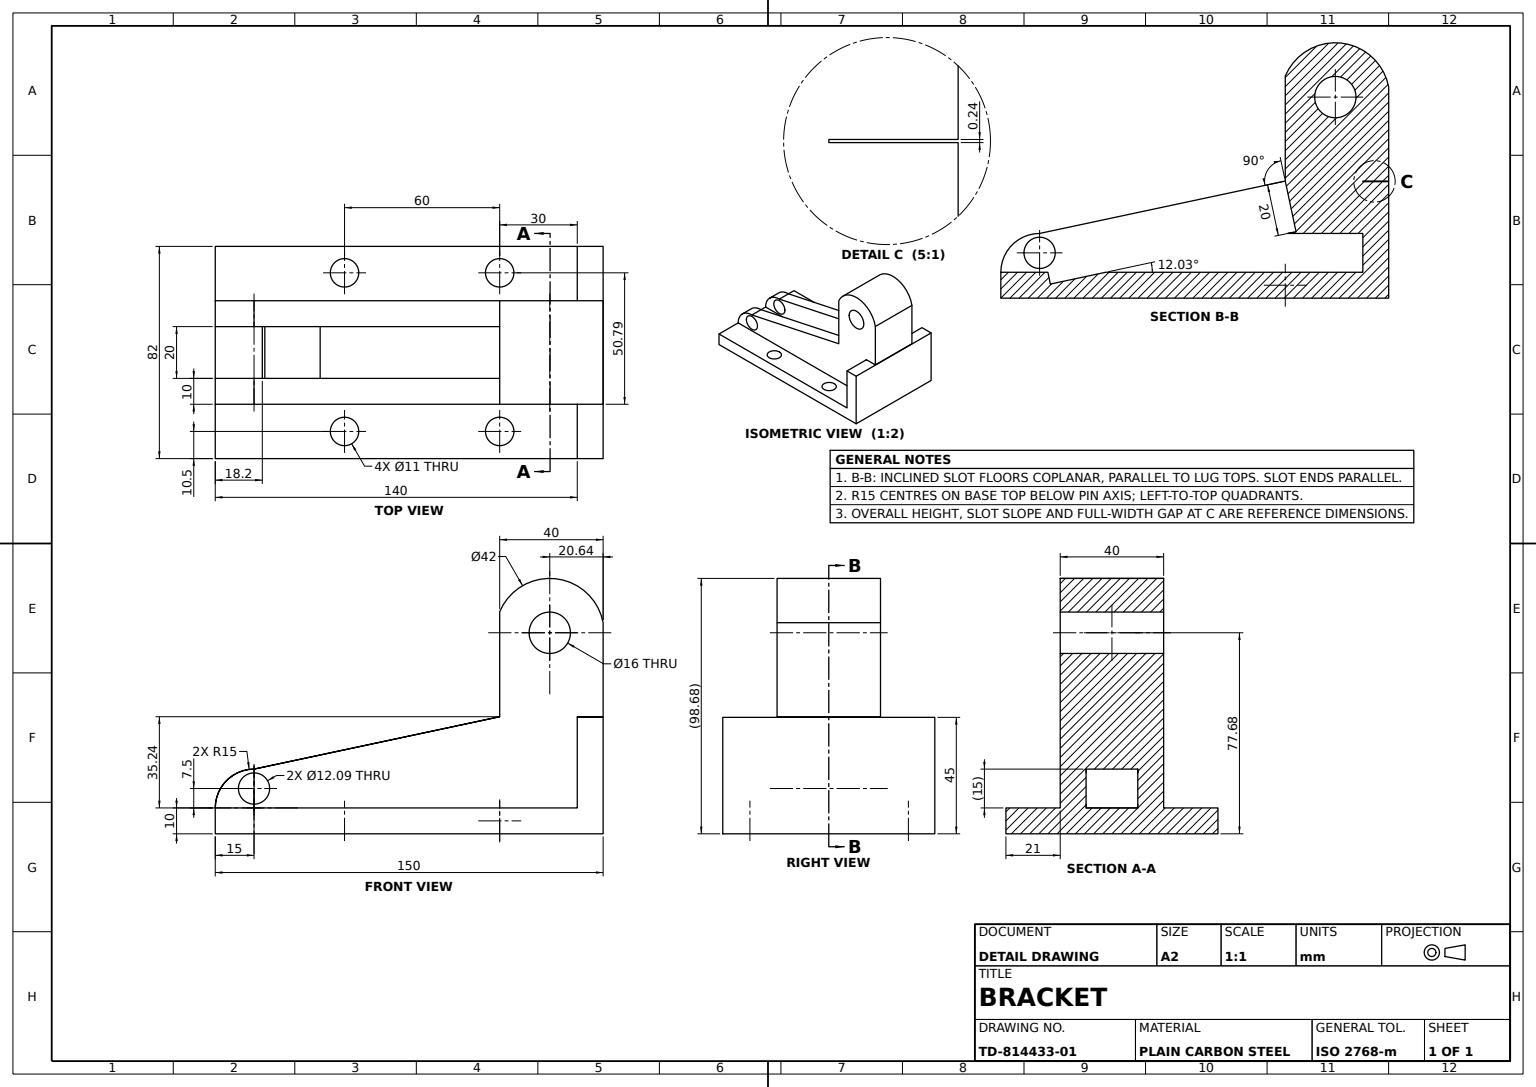
from build123d import *
from build123d.topology import SkipClean

# Parameters (mm, degrees)
BASE_ANGLE_PLATE_DEPTH           = 41
FORK_LUG_SKETCH_W                = 140
FORK_LUG_SKETCH_H                = 10
FORK_LUGS_DEPTH                  = 15
LUG_END_FILLET_R15_R             = 15
LUG_PIN_HOLE_SKETCH_R            = 6.045758047
LUG_PIN_HOLE_15_DEPTH            = 80
BASE_MOUNTING_HOLES_SKETCH_R     = 5.5
BASE_MOUNTING_HOLES_SKETCH_R_2   = 5.499920343
BASE_MOUNTING_HOLES_11_DEPTH     = 80
LUG_WEB_DEPTH                    = 10
ARM_PLATE_10MM_DEPTH             = 10
ARM_EXTENSION_40MM_DEPTH         = 40
UPRIGHT_BOSS_BLOCK_SKETCH_W      = 40
UPRIGHT_BOSS_BLOCK_SKETCH_H      = 45
UPRIGHT_BOSS_BLOCK_DEPTH         = 40
BEARING_BOSS_CLEARANCE_CUT_DEPTH = 40
BEARING_BOSS_DEPTH               = 40
BOSS_SLOT_SKETCH_W               = 97.132688683
BOSS_SLOT_SKETCH_H               = 20
BOSS_SLOT_CUT_20MM_DEPTH         = 20


with BuildPart() as part:
    # Base Angle Profile Sketch → Base Angle Plate (new, symmetric)
    with BuildSketch(Plane.XY):
        Polygon((0, 0), (150, 0), (150, 45), (140, 45), (140, 10), (0, 10), align=None)
    extrude(amount=BASE_ANGLE_PLATE_DEPTH, both=True)

    # Fork Lug Sketch → Fork Lugs (add)
    with BuildSketch(Plane(origin=(0, 10, 0), x_dir=(1, 0, 0), z_dir=(0, 1, 0))):
        with Locations((70, 15)):
            Rectangle(FORK_LUG_SKETCH_W, FORK_LUG_SKETCH_H)
        with Locations((70, -15)):
            Rectangle(FORK_LUG_SKETCH_W, FORK_LUG_SKETCH_H)
    extrude(amount=FORK_LUGS_DEPTH)

    # Lug End Fillet R15
    lug_end_fillet_r15_edges = [part.edges().sort_by_distance(p)[0] for p in [
        (0, 25, -15),
        (0, 25, 15),
    ]]
    fillet(lug_end_fillet_r15_edges, radius=LUG_END_FILLET_R15_R)

    # Lug Pin Hole Sketch → Lug Pin Hole _15 (cut)
    with BuildSketch(Plane.XY.offset(20)):
        with Locations((15, 17.5)):
            Circle(LUG_PIN_HOLE_SKETCH_R)
    extrude(amount=-LUG_PIN_HOLE_15_DEPTH, mode=Mode.SUBTRACT)

    # Base Mounting Holes Sketch → Base Mounting Holes _11 (cut)
    with BuildSketch(Plane(origin=(0, 10, 0), x_dir=(1, 0, 0), z_dir=(0, 1, 0))):
        with Locations(Location((110, -30.5, 0), (0, 0, 270))):
            Circle(BASE_MOUNTING_HOLES_SKETCH_R)
        with Locations(Location((50, -30.5, 0), (0, 0, 270))):
            Circle(BASE_MOUNTING_HOLES_SKETCH_R)
        with Locations(Location((110, 30.788589269, 0), (0, 0, 270))):
            Circle(BASE_MOUNTING_HOLES_SKETCH_R)
        with Locations(Location((50, 30.788589269, 0), (0, 0, 270))):
            Circle(BASE_MOUNTING_HOLES_SKETCH_R_2)
    extrude(amount=-BASE_MOUNTING_HOLES_11_DEPTH, mode=Mode.SUBTRACT)

    # Lug Web Sketch → Lug Web (add)
    with BuildSketch(Plane.XY.offset(20)):
        Polygon((109.382207464, 25), (109.382207464, 45), (15, 25), align=None)
    extrude(amount=-LUG_WEB_DEPTH)

    # Arm Profile Sketch → Arm Plate 10mm (add)
    with BuildSketch(Plane(origin=(0, 0, -20), x_dir=(-1, 0, 0), z_dir=(0, 0, -1))):
        Polygon((-140, 25), (-140, 45.242509992), (-110, 45.242509992), (-15, 25), align=None)
    extrude(amount=-ARM_PLATE_10MM_DEPTH)

    # Sketch17_3 → Arm Extension 40mm (add)
    with BuildSketch(Plane(origin=(0, 0, -20), x_dir=(-1, 0, 0), z_dir=(0, 0, -1))):
        Polygon((-140, 25), (-140, 45.242509992), (-110, 45.242509992), (-15, 25), align=None)
    extrude(amount=-ARM_EXTENSION_40MM_DEPTH)

    # Upright Boss Block Sketch → Upright Boss Block (add)
    with BuildSketch(Plane(origin=(110, 45.242509992, 20), x_dir=(-1, 0, 0), z_dir=(0, 0, -1))):
        with Locations((-20, 22.5)):
            Rectangle(UPRIGHT_BOSS_BLOCK_SKETCH_W, UPRIGHT_BOSS_BLOCK_SKETCH_H)
    extrude(amount=UPRIGHT_BOSS_BLOCK_DEPTH)

    # Bearing Boss Sketch → Bearing Boss Clearance Cut (cut)
    with BuildSketch(Plane.XY.offset(20)):
        with BuildLine():
            Line((137.363208202, 77.68412768), (129.363208202, 77.68412768))
            Line((129.363208202, 77.68412768), (121.363208202, 77.68412768))
            ThreePointArc((121.363208202, 77.68412768), (129.363208202, 69.68412768), (137.363208202, 77.68412768))
        make_face()
        with BuildLine():
            Line((121.363208202, 77.68412768), (129.363208202, 77.68412768))
            Line((129.363208202, 77.68412768), (137.363208202, 77.68412768))
            ThreePointArc((137.363208202, 77.68412768), (129.363208202, 85.68412768), (121.363208202, 77.68412768))
        make_face()
        with BuildLine():
            Line((137.363208202, 77.68412768), (129.363208202, 77.68412768))
            Line((129.363208202, 77.68412768), (121.363208202, 77.68412768))
            ThreePointArc((121.363208202, 77.68412768), (129.363208202, 69.68412768), (137.363208202, 77.68412768))
        make_face()
        with BuildLine():
            Line((121.363208202, 77.68412768), (129.363208202, 77.68412768))
            Line((129.363208202, 77.68412768), (137.363208202, 77.68412768))
            ThreePointArc((137.363208202, 77.68412768), (129.363208202, 85.68412768), (121.363208202, 77.68412768))
        make_face()
        with BuildLine():
            Line((110, 90.242509992), (110, 85.812237431))
            ThreePointArc((110, 85.812237431), (111.130972734, 88.104568642), (112.532075332, 90.242509992))
            Line((112.532075332, 90.242509992), (110, 90.242509992))
        make_face()
        with BuildLine():
            ThreePointArc((146.194341072, 90.242509992), (148.592137613, 86.12499693), (150, 81.572935245))
            Line((150, 81.572935245), (150, 90.242509992))
            Line((150, 90.242509992), (146.194341072, 90.242509992))
        make_face()
    extrude(amount=-BEARING_BOSS_CLEARANCE_CUT_DEPTH, mode=Mode.SUBTRACT)

    # Sketch20_3 → Bearing Boss (add)
    with SkipClean():  # the faces are left unmerged after this step: merging them gives an invalid solid
        with BuildSketch(Plane.XY.offset(20)):
            with BuildLine():
                ThreePointArc((146.194341072, 90.242509992), (129.363208202, 98.68412768), (112.532075332, 90.242509992))
                Line((112.532075332, 90.242509992), (146.194341072, 90.242509992))
            make_face()
        extrude(amount=-BEARING_BOSS_DEPTH)

    # Boss Slot Sketch → Boss Slot Cut 20mm (cut)
    with SkipClean():  # the faces are left unmerged after this step: merging them gives an invalid solid
        with BuildSketch(Plane(origin=(-4.444159319, 20.856856955, 0), x_dir=(0.9780435534944176, 0.20840059373238926, 0), z_dir=(-0.20840059373238926, 0.9780435534944176, 0))):
            with Locations((68.447012488, 0)):
                Rectangle(BOSS_SLOT_SKETCH_W, BOSS_SLOT_SKETCH_H)
        extrude(amount=-BOSS_SLOT_CUT_20MM_DEPTH, mode=Mode.SUBTRACT)


solid = part.part
